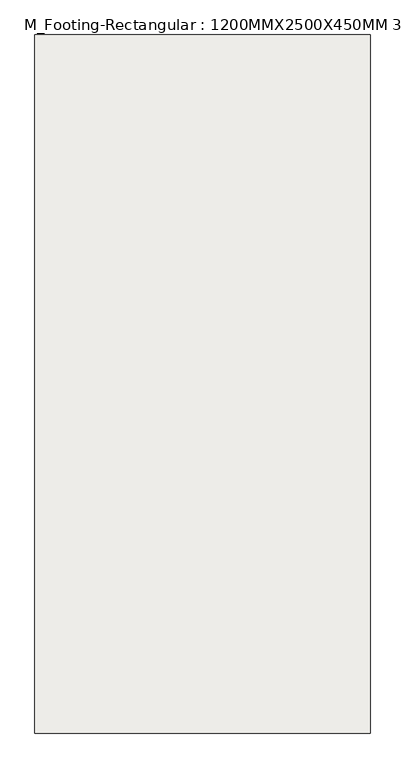
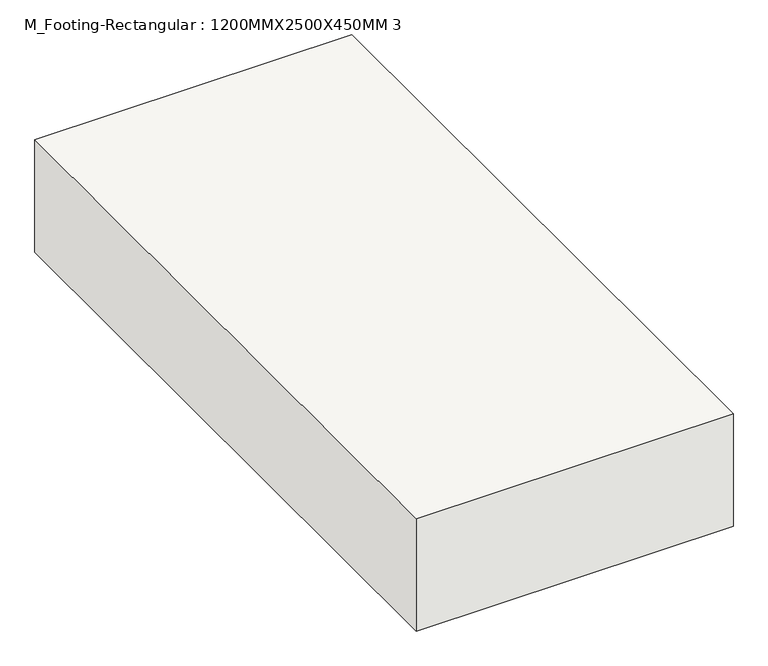
"""IFC4 building model written with IfcOpenShell, lengths in millimetres: slab geometry, M_Footing-Rectangular : 1200MMX2500X450MM 3."""

from ifc_helpers import new_model, si_unit, frame, origin, place, context, project, spatial, polyline, outline, extrude, source, transform, mapped, element, save


def m_footing_rectangular_1200mmx2500x450mm_3_75a58447(model_context):
    return source(origin(), model_context, "Body", "SweptSolid", [
        extrude(outline(polyline([(600.0, 1250.0), (600.0, -1250.0), (-600.0, -1250.0), (-600.0, 1250.0), (600.0, 1250.0)])), frame((0.0, 0.0, -450.0), z_axis=(0.0, 0.0, 1.0), x_axis=(1.0, 0.0, 0.0)), (0.0, 0.0, 1.0), 450.0),
    ])


if __name__ == "__main__":
    model = new_model("IFC4")
    model_context = context("Model", 3, world=origin())
    ifc_project = project(units=[si_unit("LENGTHUNIT", "METRE", prefix="MILLI")], contexts=[model_context])
    site = spatial("IfcSite", under=ifc_project)
    building = spatial("IfcBuilding", under=site)
    placement = place(None, origin())
    m_footing_rectangular_1200mmx2500x450mm_3_shape = m_footing_rectangular_1200mmx2500x450mm_3_75a58447(model_context)
    element("IfcSlab", 1, ObjectType="M_Footing-Rectangular : 1200MMX2500X450MM 3", at=placement, inside=building, context=model_context, shape_type="MappedRepresentation", body=[
        mapped(m_footing_rectangular_1200mmx2500x450mm_3_shape, transform((0.0, 0.0, 0.0), x_axis=(1.0, 0.0, 0.0), y_axis=(0.0, 1.0, 0.0), z_axis=(0.0, 0.0, 1.0))),
    ])
    save(model, "model.ifc")

# Revit data of these elements
# Type "M_Footing-Rectangular : 1200MMX2500X450MM 3"
#   Width = 1200 mm
#   Length = 2500 mm
#   Foundation Thickness = 450 mm
#   Structural Material [instance default] = Concrete, Cast-in-Place gray
#   Assembly Code = ""
# Element 1 (IfcSlab, "M_Footing-Rectangular : 1200MMX2500X450MM 3")
#   Materials on its faces: "Concrete, Cast-in-Place gray"
# Materials
#   "Concrete, Cast-in-Place gray": class "Concrete", colour RGB 192 192 192, transparency 0, Description = "Cast-in-place concrete", Cost = 0
